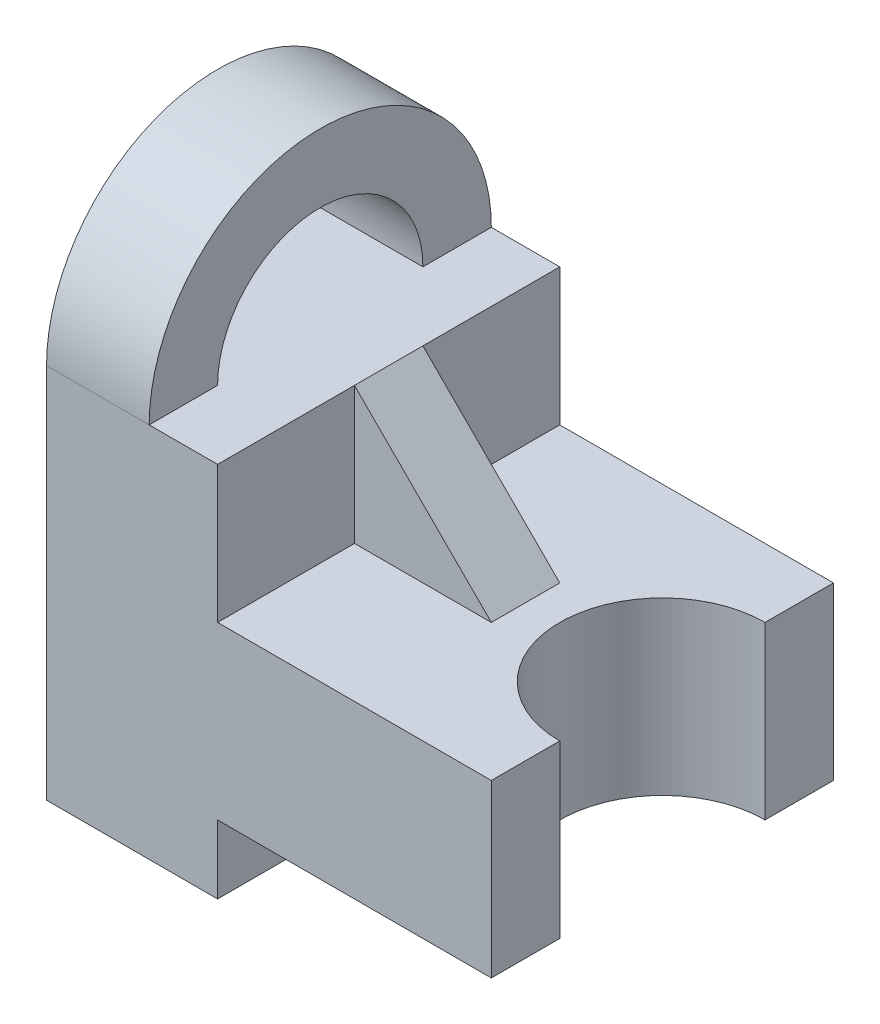
ISO-10303-21;
HEADER;
FILE_DESCRIPTION(('STEP AP214'),'2;1');
FILE_NAME('part.step','',(''),(''),'','','');
FILE_SCHEMA(('AUTOMOTIVE_DESIGN { 1 0 10303 214 1 1 1 1 }'));
ENDSEC;
DATA;
#1=APPLICATION_CONTEXT('core data for automotive mechanical design processes');
#2=APPLICATION_PROTOCOL_DEFINITION('international standard','automotive_design',2000,#1);
#3=PRODUCT_CONTEXT('',#1,'mechanical');
#4=PRODUCT('Part','Part','',(#3));
#5=PRODUCT_RELATED_PRODUCT_CATEGORY('part','',(#4));
#6=PRODUCT_DEFINITION_FORMATION('','',#4);
#7=PRODUCT_DEFINITION_CONTEXT('part definition',#1,'design');
#8=PRODUCT_DEFINITION('design','',#6,#7);
#9=PRODUCT_DEFINITION_SHAPE('','',#8);
#10=(LENGTH_UNIT() NAMED_UNIT(*) SI_UNIT(.MILLI.,.METRE.));
#11=(NAMED_UNIT(*) PLANE_ANGLE_UNIT() SI_UNIT($,.RADIAN.));
#12=(NAMED_UNIT(*) SI_UNIT($,.STERADIAN.) SOLID_ANGLE_UNIT());
#13=UNCERTAINTY_MEASURE_WITH_UNIT(LENGTH_MEASURE(1.E-05),#10,'distance_accuracy_value','');
#14=(GEOMETRIC_REPRESENTATION_CONTEXT(3) GLOBAL_UNCERTAINTY_ASSIGNED_CONTEXT((#13)) GLOBAL_UNIT_ASSIGNED_CONTEXT((#10,
#11,#12)) REPRESENTATION_CONTEXT('',''));
#15=CARTESIAN_POINT('',(0.,0.,0.));
#16=DIRECTION('',(0.,0.,1.));
#17=DIRECTION('',(1.,0.,0.));
#18=AXIS2_PLACEMENT_3D('',#15,#16,#17);
#19=CARTESIAN_POINT('',(45.,25.,-50.));
#20=DIRECTION('',(0.707106781186548,0.707106781186548,0.));
#21=DIRECTION('',(-0.707106781186548,0.707106781186548,0.));
#22=AXIS2_PLACEMENT_3D('',#19,#20,#21);
#23=PLANE('',#22);
#24=DIRECTION('',(0.707106781186548,-0.707106781186548,0.));
#25=VECTOR('',#24,1.);
#26=CARTESIAN_POINT('',(45.,25.,-30.));
#27=LINE('',#26,#25);
#28=CARTESIAN_POINT('',(25.,45.,-30.));
#29=VERTEX_POINT('',#28);
#30=CARTESIAN_POINT('',(45.,25.,-30.));
#31=VERTEX_POINT('',#30);
#32=EDGE_CURVE('E167',#29,#31,#27,.T.);
#33=ORIENTED_EDGE('',*,*,#32,.F.);
#34=DIRECTION('',(0.,0.,-1.));
#35=VECTOR('',#34,1.);
#36=CARTESIAN_POINT('',(25.,45.,-50.));
#37=LINE('',#36,#35);
#38=CARTESIAN_POINT('',(25.,45.,-20.));
#39=VERTEX_POINT('',#38);
#40=EDGE_CURVE('E225',#39,#29,#37,.T.);
#41=ORIENTED_EDGE('',*,*,#40,.F.);
#42=DIRECTION('',(-0.707106781186548,0.707106781186548,0.));
#43=VECTOR('',#42,1.);
#44=CARTESIAN_POINT('',(25.,45.,-20.));
#45=LINE('',#44,#43);
#46=CARTESIAN_POINT('',(45.,25.,-20.));
#47=VERTEX_POINT('',#46);
#48=EDGE_CURVE('E180',#47,#39,#45,.T.);
#49=ORIENTED_EDGE('',*,*,#48,.F.);
#50=DIRECTION('',(0.,0.,1.));
#51=VECTOR('',#50,1.);
#52=CARTESIAN_POINT('',(45.,25.,-50.));
#53=LINE('',#52,#51);
#54=EDGE_CURVE('E58',#31,#47,#53,.T.);
#55=ORIENTED_EDGE('',*,*,#54,.F.);
#56=EDGE_LOOP('',(#33,#41,#49,#55));
#57=FACE_BOUND('',#56,.T.);
#58=ADVANCED_FACE('F44',(#57),#23,.T.);
#59=CARTESIAN_POINT('',(25.,45.,-50.));
#60=DIRECTION('',(0.,1.,0.));
#61=DIRECTION('',(0.,0.,1.));
#62=AXIS2_PLACEMENT_3D('',#59,#60,#61);
#63=PLANE('',#62);
#64=DIRECTION('',(-1.,0.,0.));
#65=VECTOR('',#64,1.);
#66=CARTESIAN_POINT('',(25.,45.,-50.));
#67=LINE('',#66,#65);
#68=CARTESIAN_POINT('',(25.,45.,-50.));
#69=VERTEX_POINT('',#68);
#70=CARTESIAN_POINT('',(15.,45.,-50.));
#71=VERTEX_POINT('',#70);
#72=EDGE_CURVE('E233',#69,#71,#67,.T.);
#73=ORIENTED_EDGE('',*,*,#72,.T.);
#74=DIRECTION('',(0.,0.,1.));
#75=VECTOR('',#74,1.);
#76=CARTESIAN_POINT('',(15.,45.,-50.));
#77=LINE('',#76,#75);
#78=CARTESIAN_POINT('',(15.,45.,-40.));
#79=VERTEX_POINT('',#78);
#80=EDGE_CURVE('E11',#71,#79,#77,.T.);
#81=ORIENTED_EDGE('',*,*,#80,.T.);
#82=DIRECTION('',(1.,0.,0.));
#83=VECTOR('',#82,1.);
#84=CARTESIAN_POINT('',(0.,45.,-40.));
#85=LINE('',#84,#83);
#86=CARTESIAN_POINT('',(0.,45.,-40.));
#87=VERTEX_POINT('',#86);
#88=EDGE_CURVE('E193',#87,#79,#85,.T.);
#89=ORIENTED_EDGE('',*,*,#88,.F.);
#90=DIRECTION('',(0.,0.,-1.));
#91=VECTOR('',#90,1.);
#92=CARTESIAN_POINT('',(0.,45.,-10.));
#93=LINE('',#92,#91);
#94=CARTESIAN_POINT('',(0.,45.,-10.));
#95=VERTEX_POINT('',#94);
#96=EDGE_CURVE('E187',#95,#87,#93,.T.);
#97=ORIENTED_EDGE('',*,*,#96,.F.);
#98=DIRECTION('',(1.,0.,0.));
#99=VECTOR('',#98,1.);
#100=CARTESIAN_POINT('',(0.,45.,-10.));
#101=LINE('',#100,#99);
#102=CARTESIAN_POINT('',(15.,45.,-10.));
#103=VERTEX_POINT('',#102);
#104=EDGE_CURVE('E188',#95,#103,#101,.T.);
#105=ORIENTED_EDGE('',*,*,#104,.T.);
#106=CARTESIAN_POINT('',(15.,45.,0.));
#107=VERTEX_POINT('',#106);
#108=EDGE_CURVE('E52',#103,#107,#77,.T.);
#109=ORIENTED_EDGE('',*,*,#108,.T.);
#110=DIRECTION('',(-1.,0.,0.));
#111=VECTOR('',#110,1.);
#112=CARTESIAN_POINT('',(25.,45.,0.));
#113=LINE('',#112,#111);
#114=CARTESIAN_POINT('',(25.,45.,0.));
#115=VERTEX_POINT('',#114);
#116=EDGE_CURVE('E237',#115,#107,#113,.T.);
#117=ORIENTED_EDGE('',*,*,#116,.F.);
#118=EDGE_CURVE('E227',#115,#39,#37,.T.);
#119=ORIENTED_EDGE('',*,*,#118,.T.);
#120=ORIENTED_EDGE('',*,*,#40,.T.);
#121=DIRECTION('',(0.,0.,-1.));
#122=VECTOR('',#121,1.);
#123=CARTESIAN_POINT('',(25.,45.,-30.));
#124=LINE('',#123,#122);
#125=EDGE_CURVE('E295',#29,#69,#124,.T.);
#126=ORIENTED_EDGE('',*,*,#125,.T.);
#127=EDGE_LOOP('',(#73,#81,#89,#97,#105,#109,#117,#119,#120,#126));
#128=FACE_BOUND('',#127,.T.);
#129=ADVANCED_FACE('F275',(#128),#63,.T.);
#130=CARTESIAN_POINT('',(65.,0.,-50.));
#131=DIRECTION('',(1.,0.,0.));
#132=DIRECTION('',(0.,0.,-1.));
#133=AXIS2_PLACEMENT_3D('',#130,#131,#132);
#134=PLANE('',#133);
#135=DIRECTION('',(0.,1.,0.));
#136=VECTOR('',#135,1.);
#137=CARTESIAN_POINT('',(65.,-25.,-40.));
#138=LINE('',#137,#136);
#139=CARTESIAN_POINT('',(65.,0.,-40.));
#140=VERTEX_POINT('',#139);
#141=CARTESIAN_POINT('',(65.,25.,-40.));
#142=VERTEX_POINT('',#141);
#143=EDGE_CURVE('E204',#140,#142,#138,.T.);
#144=ORIENTED_EDGE('',*,*,#143,.F.);
#145=DIRECTION('',(0.,0.,1.));
#146=VECTOR('',#145,1.);
#147=CARTESIAN_POINT('',(65.,0.,-50.));
#148=LINE('',#147,#146);
#149=CARTESIAN_POINT('',(65.,0.,-50.));
#150=VERTEX_POINT('',#149);
#151=EDGE_CURVE('E263',#150,#140,#148,.T.);
#152=ORIENTED_EDGE('',*,*,#151,.F.);
#153=DIRECTION('',(0.,1.,0.));
#154=VECTOR('',#153,1.);
#155=CARTESIAN_POINT('',(65.,0.,-50.));
#156=LINE('',#155,#154);
#157=CARTESIAN_POINT('',(65.,25.,-50.));
#158=VERTEX_POINT('',#157);
#159=EDGE_CURVE('E243',#150,#158,#156,.T.);
#160=ORIENTED_EDGE('',*,*,#159,.T.);
#161=DIRECTION('',(0.,0.,1.));
#162=VECTOR('',#161,1.);
#163=CARTESIAN_POINT('',(65.,25.,-50.));
#164=LINE('',#163,#162);
#165=EDGE_CURVE('E256',#158,#142,#164,.T.);
#166=ORIENTED_EDGE('',*,*,#165,.T.);
#167=EDGE_LOOP('',(#144,#152,#160,#166));
#168=FACE_BOUND('',#167,.T.);
#169=ADVANCED_FACE('F330',(#168),#134,.T.);
#170=CARTESIAN_POINT('',(65.,25.,-50.));
#171=DIRECTION('',(0.,1.,0.));
#172=DIRECTION('',(0.,0.,1.));
#173=AXIS2_PLACEMENT_3D('',#170,#171,#172);
#174=PLANE('',#173);
#175=DIRECTION('',(-1.,0.,0.));
#176=VECTOR('',#175,1.);
#177=CARTESIAN_POINT('',(65.,25.,-50.));
#178=LINE('',#177,#176);
#179=CARTESIAN_POINT('',(25.,25.,-50.));
#180=VERTEX_POINT('',#179);
#181=EDGE_CURVE('E250',#158,#180,#178,.T.);
#182=ORIENTED_EDGE('',*,*,#181,.T.);
#183=DIRECTION('',(0.,0.,-1.));
#184=VECTOR('',#183,1.);
#185=CARTESIAN_POINT('',(25.,25.,-30.));
#186=LINE('',#185,#184);
#187=CARTESIAN_POINT('',(25.,25.,-30.));
#188=VERTEX_POINT('',#187);
#189=EDGE_CURVE('E161',#188,#180,#186,.T.);
#190=ORIENTED_EDGE('',*,*,#189,.F.);
#191=DIRECTION('',(-1.,0.,0.));
#192=VECTOR('',#191,1.);
#193=CARTESIAN_POINT('',(25.,25.,-30.));
#194=LINE('',#193,#192);
#195=EDGE_CURVE('E160',#31,#188,#194,.T.);
#196=ORIENTED_EDGE('',*,*,#195,.F.);
#197=ORIENTED_EDGE('',*,*,#54,.T.);
#198=DIRECTION('',(1.,0.,0.));
#199=VECTOR('',#198,1.);
#200=CARTESIAN_POINT('',(45.,25.,-20.));
#201=LINE('',#200,#199);
#202=CARTESIAN_POINT('',(25.,25.,-20.));
#203=VERTEX_POINT('',#202);
#204=EDGE_CURVE('E294',#203,#47,#201,.T.);
#205=ORIENTED_EDGE('',*,*,#204,.F.);
#206=DIRECTION('',(0.,0.,1.));
#207=VECTOR('',#206,1.);
#208=CARTESIAN_POINT('',(25.,25.,-20.));
#209=LINE('',#208,#207);
#210=CARTESIAN_POINT('',(25.,25.,0.));
#211=VERTEX_POINT('',#210);
#212=EDGE_CURVE('E179',#203,#211,#209,.T.);
#213=ORIENTED_EDGE('',*,*,#212,.T.);
#214=DIRECTION('',(-1.,0.,0.));
#215=VECTOR('',#214,1.);
#216=CARTESIAN_POINT('',(65.,25.,0.));
#217=LINE('',#216,#215);
#218=CARTESIAN_POINT('',(65.,25.,0.));
#219=VERTEX_POINT('',#218);
#220=EDGE_CURVE('E242',#219,#211,#217,.T.);
#221=ORIENTED_EDGE('',*,*,#220,.F.);
#222=CARTESIAN_POINT('',(65.,25.,-10.));
#223=VERTEX_POINT('',#222);
#224=EDGE_CURVE('E265',#223,#219,#164,.T.);
#225=ORIENTED_EDGE('',*,*,#224,.F.);
#226=CARTESIAN_POINT('',(65.,25.,-25.));
#227=DIRECTION('',(0.,1.,0.));
#228=DIRECTION('',(0.,0.,1.));
#229=AXIS2_PLACEMENT_3D('',#226,#227,#228);
#230=CIRCLE('',#229,15.);
#231=EDGE_CURVE('E200',#142,#223,#230,.T.);
#232=ORIENTED_EDGE('',*,*,#231,.F.);
#233=ORIENTED_EDGE('',*,*,#165,.F.);
#234=EDGE_LOOP('',(#182,#190,#196,#197,#205,#213,#221,#225,#232,#233));
#235=FACE_BOUND('',#234,.T.);
#236=ADVANCED_FACE('F157',(#235),#174,.T.);
#237=CARTESIAN_POINT('',(0.,25.,-50.));
#238=DIRECTION('',(-1.,0.,0.));
#239=DIRECTION('',(0.,0.,1.));
#240=AXIS2_PLACEMENT_3D('',#237,#238,#239);
#241=PLANE('',#240);
#242=CARTESIAN_POINT('',(0.,45.,-25.));
#243=DIRECTION('',(1.,0.,0.));
#244=DIRECTION('',(0.,0.,-1.));
#245=AXIS2_PLACEMENT_3D('',#242,#243,#244);
#246=CIRCLE('',#245,15.);
#247=EDGE_CURVE('E66',#87,#95,#246,.T.);
#248=ORIENTED_EDGE('',*,*,#247,.T.);
#249=ORIENTED_EDGE('',*,*,#96,.T.);
#250=EDGE_LOOP('',(#248,#249));
#251=FACE_BOUND('',#250,.T.);
#252=DIRECTION('',(0.,-1.,0.));
#253=VECTOR('',#252,1.);
#254=CARTESIAN_POINT('',(0.,25.,0.));
#255=LINE('',#254,#253);
#256=CARTESIAN_POINT('',(0.,45.,0.));
#257=VERTEX_POINT('',#256);
#258=CARTESIAN_POINT('',(0.,-10.,0.));
#259=VERTEX_POINT('',#258);
#260=EDGE_CURVE('E234',#257,#259,#255,.T.);
#261=ORIENTED_EDGE('',*,*,#260,.F.);
#262=CARTESIAN_POINT('',(0.,45.,-25.));
#263=DIRECTION('',(-1.,0.,0.));
#264=DIRECTION('',(0.,0.,1.));
#265=AXIS2_PLACEMENT_3D('',#262,#263,#264);
#266=CIRCLE('',#265,25.);
#267=CARTESIAN_POINT('',(0.,45.,-50.));
#268=VERTEX_POINT('',#267);
#269=EDGE_CURVE('E191',#257,#268,#266,.T.);
#270=ORIENTED_EDGE('',*,*,#269,.T.);
#271=DIRECTION('',(0.,-1.,0.));
#272=VECTOR('',#271,1.);
#273=CARTESIAN_POINT('',(0.,25.,-50.));
#274=LINE('',#273,#272);
#275=CARTESIAN_POINT('',(0.,-10.,-50.));
#276=VERTEX_POINT('',#275);
#277=EDGE_CURVE('E239',#268,#276,#274,.T.);
#278=ORIENTED_EDGE('',*,*,#277,.T.);
#279=DIRECTION('',(0.,0.,1.));
#280=VECTOR('',#279,1.);
#281=CARTESIAN_POINT('',(0.,-10.,-50.));
#282=LINE('',#281,#280);
#283=EDGE_CURVE('E212',#276,#259,#282,.T.);
#284=ORIENTED_EDGE('',*,*,#283,.T.);
#285=EDGE_LOOP('',(#261,#270,#278,#284));
#286=FACE_BOUND('',#285,.T.);
#287=ADVANCED_FACE('F50',(#251,#286),#241,.T.);
#288=DIRECTION('',(0.,1.,0.));
#289=VECTOR('',#288,1.);
#290=CARTESIAN_POINT('',(65.,-25.,-10.));
#291=LINE('',#290,#289);
#292=CARTESIAN_POINT('',(65.,0.,-10.));
#293=VERTEX_POINT('',#292);
#294=EDGE_CURVE('E205',#223,#293,#291,.F.);
#295=ORIENTED_EDGE('',*,*,#294,.F.);
#296=ORIENTED_EDGE('',*,*,#224,.T.);
#297=DIRECTION('',(0.,1.,0.));
#298=VECTOR('',#297,1.);
#299=CARTESIAN_POINT('',(65.,0.,0.));
#300=LINE('',#299,#298);
#301=CARTESIAN_POINT('',(65.,0.,0.));
#302=VERTEX_POINT('',#301);
#303=EDGE_CURVE('E255',#302,#219,#300,.T.);
#304=ORIENTED_EDGE('',*,*,#303,.F.);
#305=EDGE_CURVE('E249',#293,#302,#148,.T.);
#306=ORIENTED_EDGE('',*,*,#305,.F.);
#307=EDGE_LOOP('',(#295,#296,#304,#306));
#308=FACE_BOUND('',#307,.T.);
#309=ADVANCED_FACE('F335',(#308),#134,.T.);
#310=CARTESIAN_POINT('',(0.,0.,-50.));
#311=DIRECTION('',(0.,-1.,0.));
#312=DIRECTION('',(0.,0.,-1.));
#313=AXIS2_PLACEMENT_3D('',#310,#311,#312);
#314=PLANE('',#313);
#315=CARTESIAN_POINT('',(65.,0.,-25.));
#316=DIRECTION('',(0.,-1.,0.));
#317=DIRECTION('',(0.,0.,-1.));
#318=AXIS2_PLACEMENT_3D('',#315,#316,#317);
#319=CIRCLE('',#318,15.);
#320=EDGE_CURVE('E261',#293,#140,#319,.T.);
#321=ORIENTED_EDGE('',*,*,#320,.F.);
#322=ORIENTED_EDGE('',*,*,#305,.T.);
#323=DIRECTION('',(1.,0.,0.));
#324=VECTOR('',#323,1.);
#325=CARTESIAN_POINT('',(0.,0.,0.));
#326=LINE('',#325,#324);
#327=CARTESIAN_POINT('',(25.,0.,0.));
#328=VERTEX_POINT('',#327);
#329=EDGE_CURVE('E253',#328,#302,#326,.T.);
#330=ORIENTED_EDGE('',*,*,#329,.F.);
#331=DIRECTION('',(0.,0.,1.));
#332=VECTOR('',#331,1.);
#333=CARTESIAN_POINT('',(25.,0.,-50.));
#334=LINE('',#333,#332);
#335=CARTESIAN_POINT('',(25.,0.,-50.));
#336=VERTEX_POINT('',#335);
#337=EDGE_CURVE('E218',#336,#328,#334,.T.);
#338=ORIENTED_EDGE('',*,*,#337,.F.);
#339=DIRECTION('',(1.,0.,0.));
#340=VECTOR('',#339,1.);
#341=CARTESIAN_POINT('',(0.,0.,-50.));
#342=LINE('',#341,#340);
#343=EDGE_CURVE('E241',#336,#150,#342,.T.);
#344=ORIENTED_EDGE('',*,*,#343,.T.);
#345=ORIENTED_EDGE('',*,*,#151,.T.);
#346=EDGE_LOOP('',(#321,#322,#330,#338,#344,#345));
#347=FACE_BOUND('',#346,.T.);
#348=ADVANCED_FACE('F323',(#347),#314,.T.);
#349=CARTESIAN_POINT('',(0.,0.,-50.));
#350=DIRECTION('',(0.,0.,1.));
#351=DIRECTION('',(1.,0.,0.));
#352=AXIS2_PLACEMENT_3D('',#349,#350,#351);
#353=PLANE('',#352);
#354=ORIENTED_EDGE('',*,*,#72,.F.);
#355=DIRECTION('',(0.,1.,0.));
#356=VECTOR('',#355,1.);
#357=CARTESIAN_POINT('',(25.,45.,-50.));
#358=LINE('',#357,#356);
#359=EDGE_CURVE('E174',#180,#69,#358,.T.);
#360=ORIENTED_EDGE('',*,*,#359,.F.);
#361=ORIENTED_EDGE('',*,*,#181,.F.);
#362=ORIENTED_EDGE('',*,*,#159,.F.);
#363=ORIENTED_EDGE('',*,*,#343,.F.);
#364=DIRECTION('',(0.,1.,0.));
#365=VECTOR('',#364,1.);
#366=CARTESIAN_POINT('',(25.,-10.,-50.));
#367=LINE('',#366,#365);
#368=CARTESIAN_POINT('',(25.,-10.,-50.));
#369=VERTEX_POINT('',#368);
#370=EDGE_CURVE('E209',#369,#336,#367,.T.);
#371=ORIENTED_EDGE('',*,*,#370,.F.);
#372=DIRECTION('',(1.,0.,0.));
#373=VECTOR('',#372,1.);
#374=CARTESIAN_POINT('',(0.,-10.,-50.));
#375=LINE('',#374,#373);
#376=EDGE_CURVE('E210',#276,#369,#375,.T.);
#377=ORIENTED_EDGE('',*,*,#376,.F.);
#378=ORIENTED_EDGE('',*,*,#277,.F.);
#379=EDGE_CURVE('E232',#71,#268,#67,.T.);
#380=ORIENTED_EDGE('',*,*,#379,.F.);
#381=EDGE_LOOP('',(#354,#360,#361,#362,#363,#371,#377,#378,#380));
#382=FACE_BOUND('',#381,.T.);
#383=ADVANCED_FACE('F310',(#382),#353,.F.);
#384=CARTESIAN_POINT('',(0.,0.,0.));
#385=DIRECTION('',(0.,0.,1.));
#386=DIRECTION('',(1.,0.,0.));
#387=AXIS2_PLACEMENT_3D('',#384,#385,#386);
#388=PLANE('',#387);
#389=DIRECTION('',(0.,-1.,0.));
#390=VECTOR('',#389,1.);
#391=CARTESIAN_POINT('',(25.,25.,0.));
#392=LINE('',#391,#390);
#393=EDGE_CURVE('E286',#115,#211,#392,.T.);
#394=ORIENTED_EDGE('',*,*,#393,.F.);
#395=ORIENTED_EDGE('',*,*,#116,.T.);
#396=EDGE_CURVE('E230',#107,#257,#113,.T.);
#397=ORIENTED_EDGE('',*,*,#396,.T.);
#398=ORIENTED_EDGE('',*,*,#260,.T.);
#399=DIRECTION('',(1.,0.,0.));
#400=VECTOR('',#399,1.);
#401=CARTESIAN_POINT('',(0.,-10.,0.));
#402=LINE('',#401,#400);
#403=CARTESIAN_POINT('',(25.,-10.,0.));
#404=VERTEX_POINT('',#403);
#405=EDGE_CURVE('E206',#259,#404,#402,.T.);
#406=ORIENTED_EDGE('',*,*,#405,.T.);
#407=DIRECTION('',(0.,1.,0.));
#408=VECTOR('',#407,1.);
#409=CARTESIAN_POINT('',(25.,-10.,0.));
#410=LINE('',#409,#408);
#411=EDGE_CURVE('E211',#404,#328,#410,.T.);
#412=ORIENTED_EDGE('',*,*,#411,.T.);
#413=ORIENTED_EDGE('',*,*,#329,.T.);
#414=ORIENTED_EDGE('',*,*,#303,.T.);
#415=ORIENTED_EDGE('',*,*,#220,.T.);
#416=EDGE_LOOP('',(#394,#395,#397,#398,#406,#412,#413,#414,#415));
#417=FACE_BOUND('',#416,.T.);
#418=ADVANCED_FACE('F288',(#417),#388,.T.);
#419=CARTESIAN_POINT('',(25.,-10.,-50.));
#420=DIRECTION('',(1.,0.,0.));
#421=DIRECTION('',(0.,0.,-1.));
#422=AXIS2_PLACEMENT_3D('',#419,#420,#421);
#423=PLANE('',#422);
#424=ORIENTED_EDGE('',*,*,#411,.F.);
#425=DIRECTION('',(0.,0.,1.));
#426=VECTOR('',#425,1.);
#427=CARTESIAN_POINT('',(25.,-10.,-50.));
#428=LINE('',#427,#426);
#429=EDGE_CURVE('E224',#369,#404,#428,.T.);
#430=ORIENTED_EDGE('',*,*,#429,.F.);
#431=ORIENTED_EDGE('',*,*,#370,.T.);
#432=ORIENTED_EDGE('',*,*,#337,.T.);
#433=EDGE_LOOP('',(#424,#430,#431,#432));
#434=FACE_BOUND('',#433,.T.);
#435=ADVANCED_FACE('F319',(#434),#423,.T.);
#436=CARTESIAN_POINT('',(0.,-10.,-50.));
#437=DIRECTION('',(0.,-1.,0.));
#438=DIRECTION('',(0.,0.,-1.));
#439=AXIS2_PLACEMENT_3D('',#436,#437,#438);
#440=PLANE('',#439);
#441=ORIENTED_EDGE('',*,*,#405,.F.);
#442=ORIENTED_EDGE('',*,*,#283,.F.);
#443=ORIENTED_EDGE('',*,*,#376,.T.);
#444=ORIENTED_EDGE('',*,*,#429,.T.);
#445=EDGE_LOOP('',(#441,#442,#443,#444));
#446=FACE_BOUND('',#445,.T.);
#447=ADVANCED_FACE('F320',(#446),#440,.T.);
#448=CARTESIAN_POINT('',(65.,-25.,-25.));
#449=DIRECTION('',(0.,1.,0.));
#450=DIRECTION('',(0.,0.,1.));
#451=AXIS2_PLACEMENT_3D('',#448,#449,#450);
#452=CYLINDRICAL_SURFACE('',#451,15.);
#453=ORIENTED_EDGE('',*,*,#143,.T.);
#454=ORIENTED_EDGE('',*,*,#231,.T.);
#455=ORIENTED_EDGE('',*,*,#294,.T.);
#456=ORIENTED_EDGE('',*,*,#320,.T.);
#457=EDGE_LOOP('',(#453,#454,#455,#456));
#458=FACE_BOUND('',#457,.T.);
#459=ADVANCED_FACE('F362',(#458),#452,.F.);
#460=CARTESIAN_POINT('',(15.,45.,-25.));
#461=DIRECTION('',(-1.,0.,0.));
#462=DIRECTION('',(0.,0.,1.));
#463=AXIS2_PLACEMENT_3D('',#460,#461,#462);
#464=CYLINDRICAL_SURFACE('',#463,25.);
#465=CARTESIAN_POINT('',(15.,45.,-25.));
#466=DIRECTION('',(-1.,0.,0.));
#467=DIRECTION('',(0.,0.,1.));
#468=AXIS2_PLACEMENT_3D('',#465,#466,#467);
#469=CIRCLE('',#468,25.);
#470=EDGE_CURVE('E198',#107,#71,#469,.T.);
#471=ORIENTED_EDGE('',*,*,#470,.T.);
#472=ORIENTED_EDGE('',*,*,#379,.T.);
#473=ORIENTED_EDGE('',*,*,#269,.F.);
#474=ORIENTED_EDGE('',*,*,#396,.F.);
#475=EDGE_LOOP('',(#471,#472,#473,#474));
#476=FACE_BOUND('',#475,.T.);
#477=ADVANCED_FACE('F276',(#476),#464,.T.);
#478=CARTESIAN_POINT('',(15.,45.,-25.));
#479=DIRECTION('',(-1.,0.,0.));
#480=DIRECTION('',(0.,0.,1.));
#481=AXIS2_PLACEMENT_3D('',#478,#479,#480);
#482=PLANE('',#481);
#483=ORIENTED_EDGE('',*,*,#108,.F.);
#484=CARTESIAN_POINT('',(15.,45.,-25.));
#485=DIRECTION('',(1.,0.,0.));
#486=DIRECTION('',(0.,0.,-1.));
#487=AXIS2_PLACEMENT_3D('',#484,#485,#486);
#488=CIRCLE('',#487,15.);
#489=EDGE_CURVE('E176',#79,#103,#488,.T.);
#490=ORIENTED_EDGE('',*,*,#489,.F.);
#491=ORIENTED_EDGE('',*,*,#80,.F.);
#492=ORIENTED_EDGE('',*,*,#470,.F.);
#493=EDGE_LOOP('',(#483,#490,#491,#492));
#494=FACE_BOUND('',#493,.T.);
#495=ADVANCED_FACE('F283',(#494),#482,.F.);
#496=CARTESIAN_POINT('',(0.,45.,-25.));
#497=DIRECTION('',(1.,0.,0.));
#498=DIRECTION('',(0.,0.,-1.));
#499=AXIS2_PLACEMENT_3D('',#496,#497,#498);
#500=CYLINDRICAL_SURFACE('',#499,15.);
#501=ORIENTED_EDGE('',*,*,#489,.T.);
#502=ORIENTED_EDGE('',*,*,#104,.F.);
#503=ORIENTED_EDGE('',*,*,#247,.F.);
#504=ORIENTED_EDGE('',*,*,#88,.T.);
#505=EDGE_LOOP('',(#501,#502,#503,#504));
#506=FACE_BOUND('',#505,.T.);
#507=ADVANCED_FACE('F350',(#506),#500,.F.);
#508=CARTESIAN_POINT('',(25.,25.,-20.));
#509=DIRECTION('',(-1.,0.,0.));
#510=DIRECTION('',(0.,0.,1.));
#511=AXIS2_PLACEMENT_3D('',#508,#509,#510);
#512=PLANE('',#511);
#513=ORIENTED_EDGE('',*,*,#393,.T.);
#514=ORIENTED_EDGE('',*,*,#212,.F.);
#515=DIRECTION('',(0.,-1.,0.));
#516=VECTOR('',#515,1.);
#517=CARTESIAN_POINT('',(25.,25.,-20.));
#518=LINE('',#517,#516);
#519=EDGE_CURVE('E292',#39,#203,#518,.T.);
#520=ORIENTED_EDGE('',*,*,#519,.F.);
#521=ORIENTED_EDGE('',*,*,#118,.F.);
#522=EDGE_LOOP('',(#513,#514,#520,#521));
#523=FACE_BOUND('',#522,.T.);
#524=ADVANCED_FACE('F333',(#523),#512,.F.);
#525=CARTESIAN_POINT('',(0.,0.,-20.));
#526=DIRECTION('',(0.,0.,1.));
#527=DIRECTION('',(1.,0.,0.));
#528=AXIS2_PLACEMENT_3D('',#525,#526,#527);
#529=PLANE('',#528);
#530=ORIENTED_EDGE('',*,*,#519,.T.);
#531=ORIENTED_EDGE('',*,*,#204,.T.);
#532=ORIENTED_EDGE('',*,*,#48,.T.);
#533=EDGE_LOOP('',(#530,#531,#532));
#534=FACE_BOUND('',#533,.T.);
#535=ADVANCED_FACE('F337',(#534),#529,.T.);
#536=CARTESIAN_POINT('',(25.,45.,-30.));
#537=DIRECTION('',(-1.,0.,0.));
#538=DIRECTION('',(0.,0.,1.));
#539=AXIS2_PLACEMENT_3D('',#536,#537,#538);
#540=PLANE('',#539);
#541=ORIENTED_EDGE('',*,*,#359,.T.);
#542=ORIENTED_EDGE('',*,*,#125,.F.);
#543=DIRECTION('',(0.,1.,0.));
#544=VECTOR('',#543,1.);
#545=CARTESIAN_POINT('',(25.,45.,-30.));
#546=LINE('',#545,#544);
#547=EDGE_CURVE('E164',#188,#29,#546,.T.);
#548=ORIENTED_EDGE('',*,*,#547,.F.);
#549=ORIENTED_EDGE('',*,*,#189,.T.);
#550=EDGE_LOOP('',(#541,#542,#548,#549));
#551=FACE_BOUND('',#550,.T.);
#552=ADVANCED_FACE('F302',(#551),#540,.F.);
#553=CARTESIAN_POINT('',(0.,0.,-30.));
#554=DIRECTION('',(0.,0.,1.));
#555=DIRECTION('',(1.,0.,0.));
#556=AXIS2_PLACEMENT_3D('',#553,#554,#555);
#557=PLANE('',#556);
#558=ORIENTED_EDGE('',*,*,#32,.T.);
#559=ORIENTED_EDGE('',*,*,#195,.T.);
#560=ORIENTED_EDGE('',*,*,#547,.T.);
#561=EDGE_LOOP('',(#558,#559,#560));
#562=FACE_BOUND('',#561,.T.);
#563=ADVANCED_FACE('F166',(#562),#557,.F.);
#564=CLOSED_SHELL('',(#58,#129,#169,#236,#287,#309,#348,#383,#418,#435,#447,#459,#477,#495,#507,
#524,#535,#552,#563));
#565=MANIFOLD_SOLID_BREP('B2',#564);
#566=ADVANCED_BREP_SHAPE_REPRESENTATION('',(#18,#565),#14);
#567=SHAPE_DEFINITION_REPRESENTATION(#9,#566);
ENDSEC;
END-ISO-10303-21;
